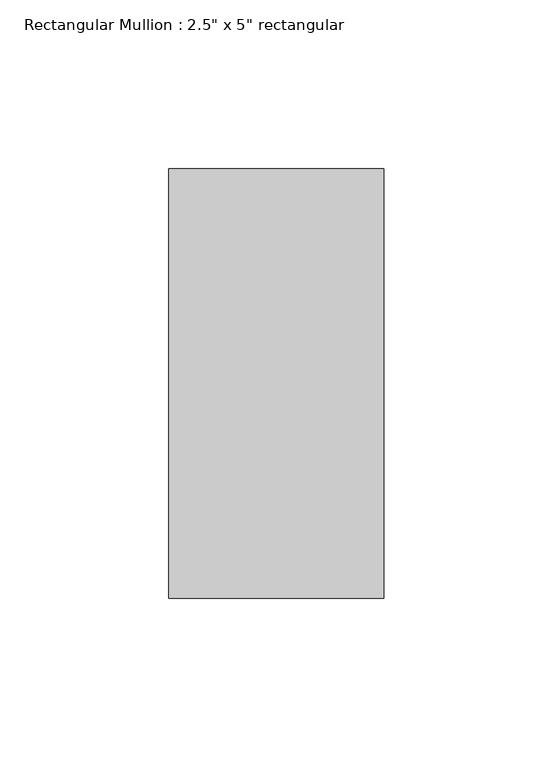
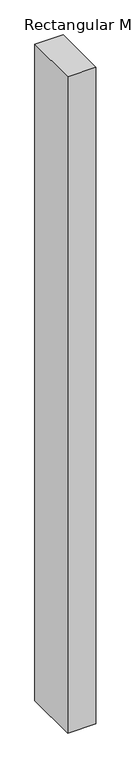
"""IFC4 building model written with IfcOpenShell, lengths in millimetres: member geometry."""

from ifc_helpers import new_model, si_unit, frame, origin, place, context, project, spatial, polyline, outline, extrude, source, transform, mapped, element, save


def member_20042e51(model_context):
    return source(origin(), model_context, "Body", "SweptSolid", [
        extrude(outline(polyline([(0.0, 63.5), (0.0, -63.5), (-63.5, -63.5), (-63.5, 63.5), (0.0, 63.5)])), frame((0.0, 0.0, -1556.7181357), z_axis=(0.0, 0.0, 1.0), x_axis=(1.0, 0.0, 0.0)), (0.0, 0.0, 1.0), 1556.7181357),
    ])


if __name__ == "__main__":
    model = new_model("IFC4")
    model_context = context("Model", 3, world=origin())
    ifc_project = project(units=[si_unit("LENGTHUNIT", "METRE", prefix="MILLI")], contexts=[model_context])
    site = spatial("IfcSite", under=ifc_project)
    building = spatial("IfcBuilding", under=site)
    placement = place(None, origin())
    member_shape = member_20042e51(model_context)
    element("IfcMember", 1, ObjectType="Rectangular Mullion : 2.5\" x 5\" rectangular", at=placement, inside=building, context=model_context, shape_type="MappedRepresentation", body=[
        mapped(member_shape, transform((0.0, 0.0, 0.0), x_axis=(1.0, 0.0, 0.0), y_axis=(0.0, 1.0, 0.0), z_axis=(0.0, 0.0, 1.0))),
    ])
    save(model, "model.ifc")

# Revit data of these elements
# Type "Rectangular Mullion : 2.5\" x 5\" rectangular"
#   built-in parameter 1007304 = 0.416667 (stored number, unit not read)
#   built-in parameter 1007301 = 0.104167 (stored number, unit not read)
#   built-in parameter 1007300 = 0.104167 (stored number, unit not read)
# Element 1 (IfcMember, "Rectangular Mullion : 2.5\" x 5\" rectangular")
#   Materials on its faces: "Aluminum"
# Materials
#   "Aluminum": class "Metal", colour RGB 247 247 247, transparency 0, Description = "Aluminum 6061", Cost = 0
